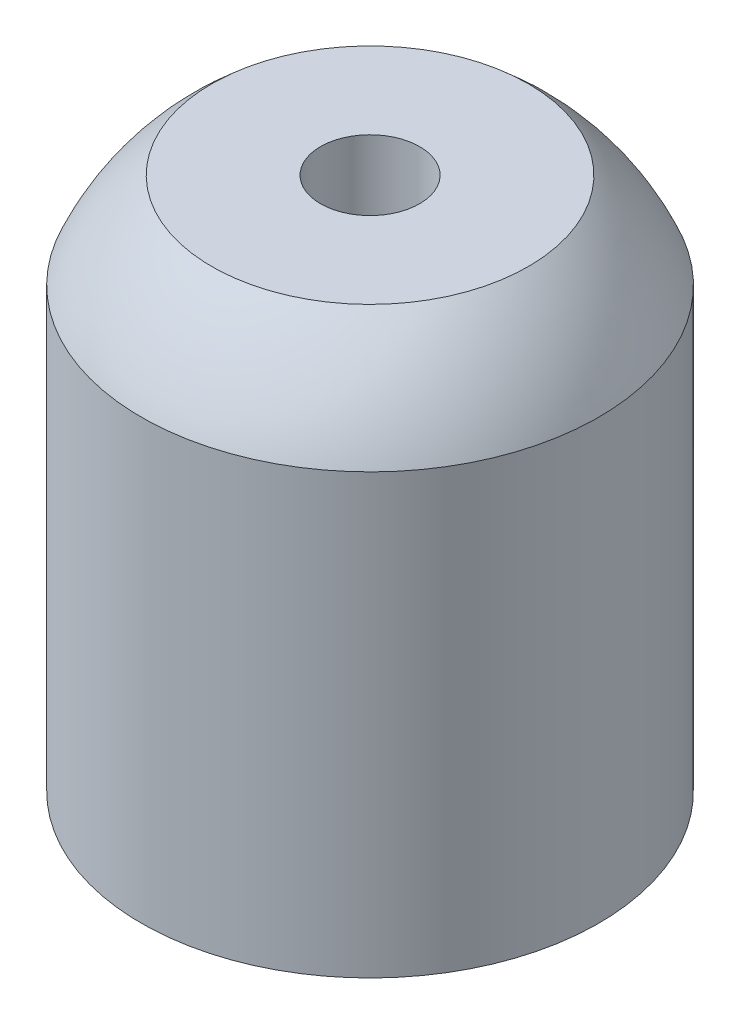
from build123d import *

# Parameters (mm, degrees)
CAP_BODY_PROFILE_SKETCH_W = 12
CAP_BODY_PROFILE_SKETCH_H = 23
TOP_DOME_8MM_FACE_RADIUS  = 12
TOP_DOME_8MM_HEIGHT       = 8
CENTRE_HOLE_SKETCH_R      = 2.6
CENTRE_HOLE_5_2X10_DEPTH  = 10


with BuildPart() as part:
    # Cap Body Profile Sketch → Cap Body _24x23 (revolve)
    with BuildSketch(Plane(origin=(0, 0, 0), x_dir=(0, 0, -1), z_dir=(1, 0, 0)), mode=Mode.PRIVATE) as cap_body_24x23_sk:
        with Locations((-6, 11.5)):
            Rectangle(CAP_BODY_PROFILE_SKETCH_W, CAP_BODY_PROFILE_SKETCH_H)
    revolve(cap_body_24x23_sk.sketch.rotate(Axis((0, 0, 0), (0, 1, 0)), 180), axis=Axis((0, 0, 0), (0, 1, 0)))

    # Top Dome 8mm: a dome of height H over a round flat face of radius A is a cap of a sphere of radius (A * A + H * H) / (2 * H)
    top_dome_8mm_r = (TOP_DOME_8MM_FACE_RADIUS * TOP_DOME_8MM_FACE_RADIUS + TOP_DOME_8MM_HEIGHT * TOP_DOME_8MM_HEIGHT) / (2 * TOP_DOME_8MM_HEIGHT)
    top_dome_8mm_base = Plane((0, 23, 0), z_dir=(0, 1, 0))
    with Locations(top_dome_8mm_base.offset(TOP_DOME_8MM_HEIGHT - top_dome_8mm_r)):
        top_dome_8mm_ball = Sphere(top_dome_8mm_r, mode=Mode.PRIVATE)
    add(split(top_dome_8mm_ball, bisect_by=top_dome_8mm_base, keep=Keep.TOP, mode=Mode.PRIVATE))

    # Dome Top Flat Trim
    split(bisect_by=Plane(origin=(0, 28, 0), x_dir=(-1, 0, 0), z_dir=(0, -1, 0)), keep=Keep.TOP)

    # Centre Hole Sketch → Centre Hole _5.2x10 (cut)
    with BuildSketch(Plane(origin=(0, 28, 0), x_dir=(1, 0, 0), z_dir=(0, 1, 0))):
        with Locations(Location((0, 0, 0), (0, 0, 270))):
            Circle(CENTRE_HOLE_SKETCH_R)
    extrude(amount=-CENTRE_HOLE_5_2X10_DEPTH, mode=Mode.SUBTRACT)


solid = part.part
